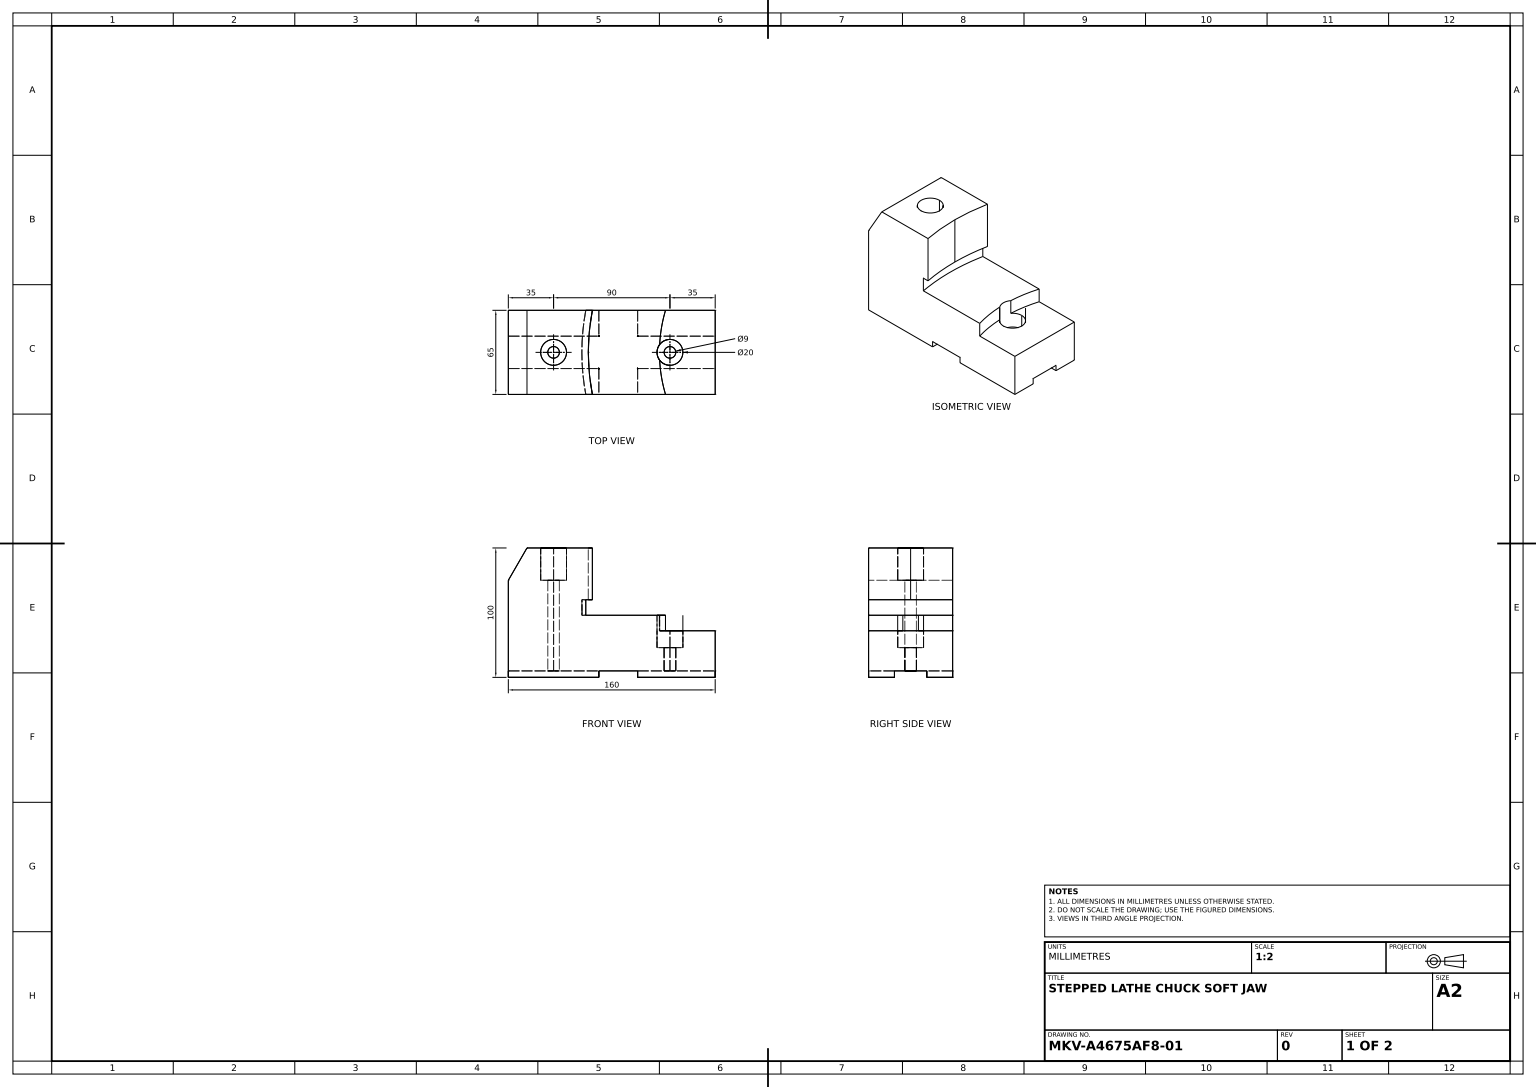
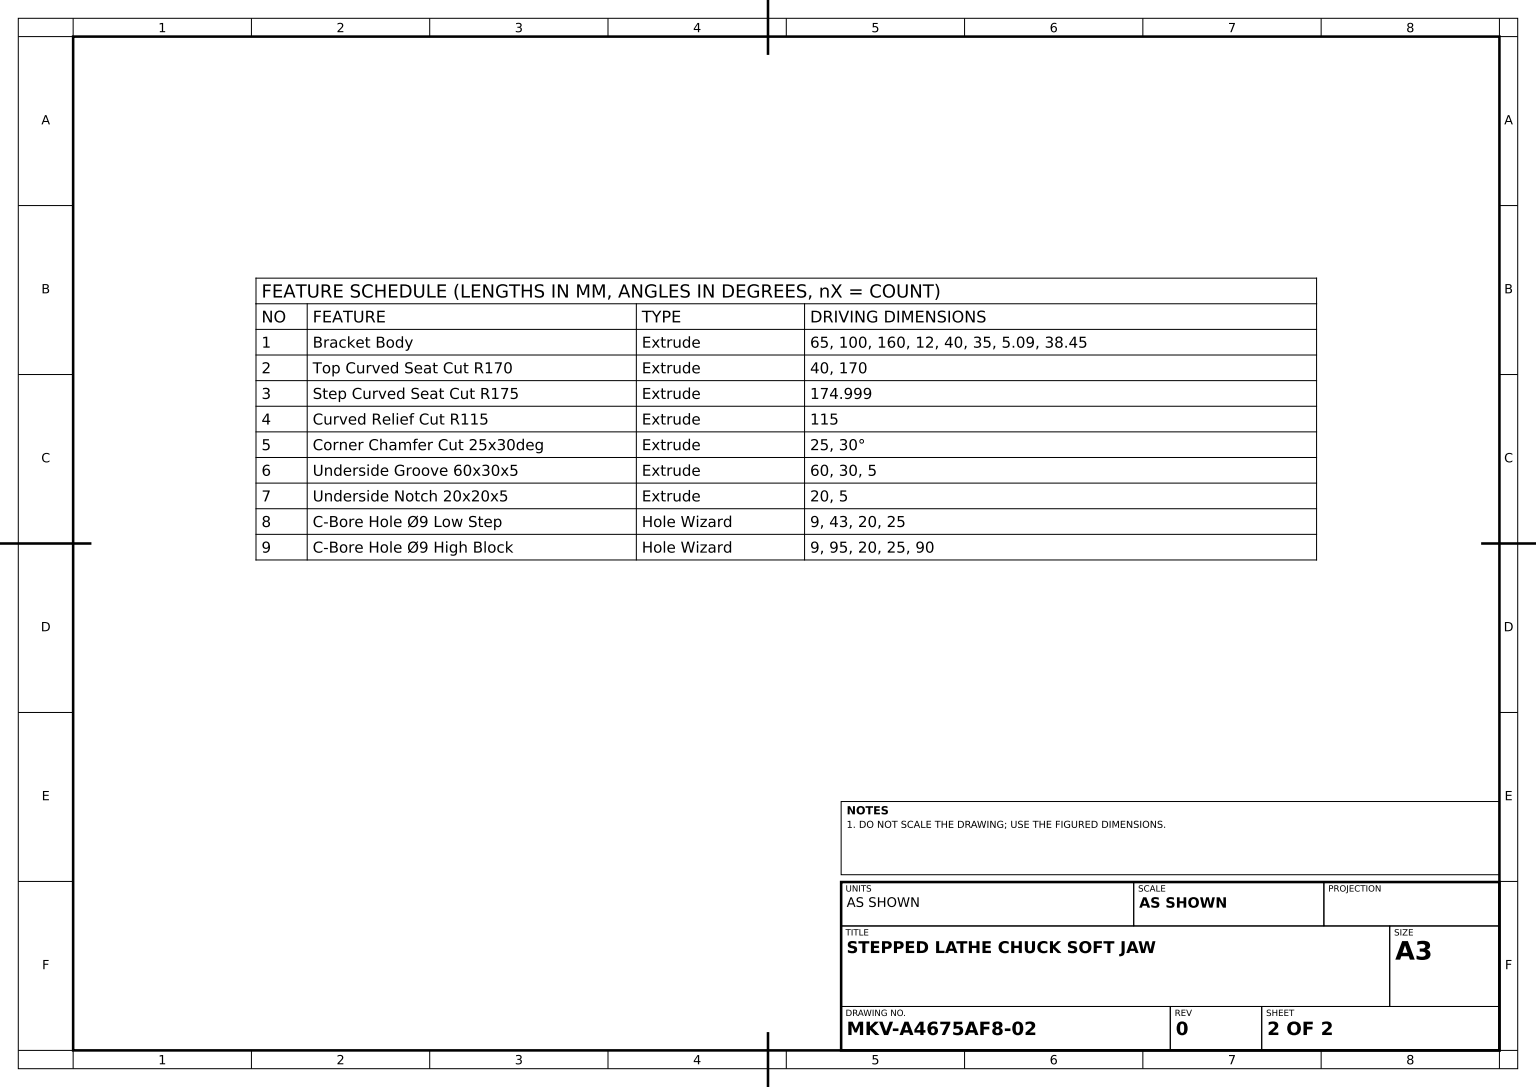
from build123d import *

# Parameters (mm, degrees)
BRACKET_BODY_DEPTH                   = 32.5
TOP_CURVED_SEAT_CUT_R170_DEPTH       = 164.343962239
TOP_CURVED_SEAT_CUT_R170_DEPTH_BACK  = 40
STEP_CURVED_SEAT_CUT_R175_DEPTH      = 12
CURVED_RELIEF_CUT_R115_DEPTH         = 12
CORNER_CHAMFER_CUT_25X30DEG_DEPTH    = 173.771525432
UNDERSIDE_GROOVE_SKETCH_60X30_W      = 30
UNDERSIDE_GROOVE_SKETCH_60X30_H      = 5
UNDERSIDE_GROOVE_60X30X5_DEPTH       = 173.771525432
UNDERSIDE_NOTCH_SKETCH_20X20_W       = 25
UNDERSIDE_NOTCH_SKETCH_20X20_H       = 5
UNDERSIDE_NOTCH_20X20X5_DEPTH        = 192.458219985
C_BORE_HOLE_9_LOW_STEP_D             = 9
C_BORE_HOLE_9_LOW_STEP_CBORE_D       = 20
C_BORE_HOLE_9_LOW_STEP_CBORE_DEPTH   = 25
C_BORE_HOLE_9_HIGH_BLOCK_D           = 9
C_BORE_HOLE_9_HIGH_BLOCK_CBORE_D     = 20
C_BORE_HOLE_9_HIGH_BLOCK_CBORE_DEPTH = 25


with BuildPart() as part:
    # Bracket Side Profile Sketch → Bracket Body (new, symmetric)
    with BuildSketch(Plane.XY):
        Polygon((35, 0), (-125, 0), (-125, 100), (-60, 100), (-60, 60), (-65.09, 60), (-65.09, 48), (-3.45, 48), (-3.45, 36), (35, 36), align=None)
    extrude(amount=BRACKET_BODY_DEPTH, both=True)

    # Top Curved Seat Sketch R170 → Top Curved Seat Cut R170 (cut, two sides: drawn at the far end of the back side and taken through both)
    with BuildSketch(Plane(origin=(0, 100, 0), x_dir=(1, 0, 0), z_dir=(0, 1, 0)).offset(-TOP_CURVED_SEAT_CUT_R170_DEPTH_BACK)):
        with BuildLine():
            ThreePointArc((-60, 32.5), (-63.13553404, 0), (-60, -32.5))
            Line((-60, -32.5), (-60, 32.5))
        make_face()
    extrude(amount=TOP_CURVED_SEAT_CUT_R170_DEPTH + TOP_CURVED_SEAT_CUT_R170_DEPTH_BACK, mode=Mode.SUBTRACT)

    # Step Curved Seat Sketch R175 → Step Curved Seat Cut R175 (cut)
    with BuildSketch(Plane(origin=(0, 48, 0), x_dir=(1, 0, 0), z_dir=(0, 1, 0))):
        with BuildLine():
            ThreePointArc((-65.09, 32.5), (-68.134357932, 0), (-65.09, -32.5))
            Line((-65.09, -32.5), (-65.09, 32.5))
        make_face()
    extrude(amount=STEP_CURVED_SEAT_CUT_R175_DEPTH, mode=Mode.SUBTRACT)

    # Curved Relief Sketch R115 → Curved Relief Cut R115 (cut)
    with BuildSketch(Plane(origin=(0, 36, 0), x_dir=(1, 0, 0), z_dir=(0, 1, 0))):
        with BuildLine():
            Line((-3.45, -32.5), (-3.45, 32.5))
            ThreePointArc((-3.45, 32.5), (-8.137942635, 0), (-3.45, -32.5))
        make_face()
    extrude(amount=CURVED_RELIEF_CUT_R115_DEPTH, mode=Mode.SUBTRACT)

    # Corner Chamfer Sketch 25x30deg → Corner Chamfer Cut 25x30deg (cut, through all)
    with BuildSketch(Plane.XY.offset(32.5)):
        Polygon((-125, 100), (-110.566242501, 100.000001332), (-125, 75), align=None)
    extrude(amount=-CORNER_CHAMFER_CUT_25X30DEG_DEPTH, mode=Mode.SUBTRACT)

    # Underside Groove Sketch 60x30 → Underside Groove 60x30x5 (cut, through all)
    with BuildSketch(Plane.XY.offset(32.5)):
        with Locations((-40, 2.5)):
            Rectangle(UNDERSIDE_GROOVE_SKETCH_60X30_W, UNDERSIDE_GROOVE_SKETCH_60X30_H)
    extrude(amount=-UNDERSIDE_GROOVE_60X30X5_DEPTH, mode=Mode.SUBTRACT)

    # Underside Notch Sketch 20x20 → Underside Notch 20x20x5 (cut, through all)
    with BuildSketch(Plane(origin=(35, 0, 0), x_dir=(0, 0, -1), z_dir=(1, 0, 0))):
        with Locations((0, 2.5)):
            Rectangle(UNDERSIDE_NOTCH_SKETCH_20X20_W, UNDERSIDE_NOTCH_SKETCH_20X20_H)
    extrude(amount=-UNDERSIDE_NOTCH_20X20X5_DEPTH, mode=Mode.SUBTRACT)

    # C-Bore Hole Ø9 Low Step (through all)
    with Locations(Plane(origin=(0, 48, 0), x_dir=(1, 0, 0), z_dir=(0, 1, 0))):
        with Locations((0, 0)):
            CounterBoreHole(C_BORE_HOLE_9_LOW_STEP_D / 2, C_BORE_HOLE_9_LOW_STEP_CBORE_D / 2, C_BORE_HOLE_9_LOW_STEP_CBORE_DEPTH)

    # C-Bore Hole Ø9 High Block (through all)
    with Locations(Plane(origin=(0, 100, 0), x_dir=(1, 0, 0), z_dir=(0, 1, 0))):
        with Locations((-90, 0)):
            CounterBoreHole(C_BORE_HOLE_9_HIGH_BLOCK_D / 2, C_BORE_HOLE_9_HIGH_BLOCK_CBORE_D / 2, C_BORE_HOLE_9_HIGH_BLOCK_CBORE_DEPTH)


solid = part.part
